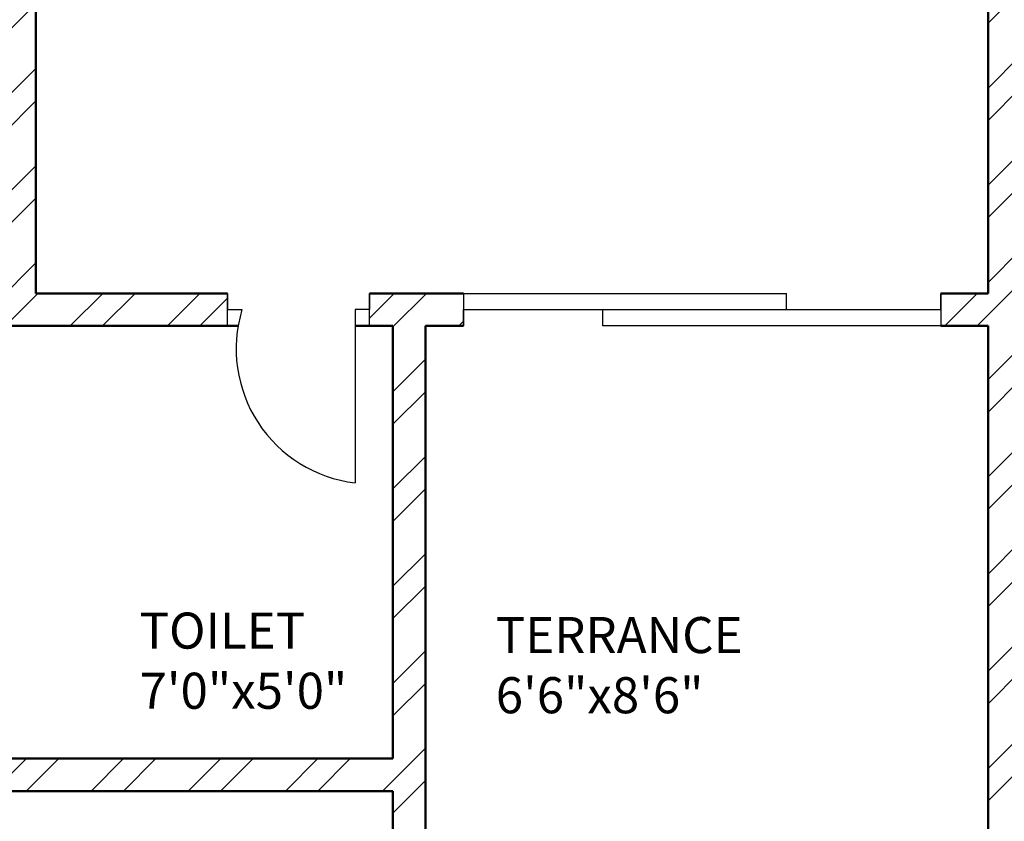
# Model space of a CAD drawing. Units: inches. Extents: x 963 to 2075, y 289 to 2657.
# Tile 5 of 98: x 1374 to 1511, y 1474 to 1585. Entities that reach past the tile are written whole.
import ezdxf

# ---------------------------------------------------------------- set-up
doc = ezdxf.new("R2010")
doc.units = ezdxf.units.IN
for name, color, linetype, lineweight in [('A-AREA-IDEN', 7, 'Continuous', 18), ('A-DOOR', 4, 'Continuous', 25), ('A-GLAZ', 3, 'Continuous', 25), ('A-WALL', 7, 'Continuous', 50), ('A-WALL-PATT', 8, 'Continuous', 13)]:
    doc.layers.add(name, color=color, linetype=linetype, lineweight=lineweight)
doc.styles.get("Standard").update_dxf_attribs({"font": 'arial.ttf'})

msp = doc.modelspace()

# ---------------------------------------------------------------- hatches: boundary and pattern name
at = {"layer": 'A-WALL-PATT'}
h = msp.add_hatch(dxfattribs=at)
h.set_pattern_fill('ANSI32', color=256)
h.paths.add_polyline_path([(1296.92, 2558.32), (1203.92, 2558.32), (1203.92, 2493.82), (1191.53, 2493.82), (1191.53, 2489.32), (1211.06, 2489.32), (1211.06, 2492.02), (1211.06, 2493.82), (1208.42, 2493.82), (1208.42, 2553.82), (1292.42, 2553.82), (1292.42, 2538.86), (1296.92, 2538.86)])
h.paths.add_polyline_path([(1442.42, 2558.32), (1349.42, 2558.32), (1349.42, 2538.94), (1353.92, 2538.94), (1353.92, 2553.82), (1437.92, 2553.82), (1437.92, 2493.82), (1434.54, 2493.82), (1434.54, 2489.32), (1448.31, 2489.32), (1448.31, 2491.57), (1448.31, 2493.82), (1442.42, 2493.82)])
h.paths.add_polyline_path([(1415.55, 2491.57), (1415.55, 2493.82), (1340.94, 2493.82), (1340.94, 2489.32), (1371.92, 2489.32), (1371.92, 2378.32), (1367.6, 2378.32), (1367.6, 2373.82), (1371.92, 2373.82), (1371.92, 2355.19), (1376.42, 2355.19), (1376.42, 2489.32), (1415.55, 2489.32)])
h.paths.add_polyline_path([(1304.94, 2491.57), (1304.94, 2493.82), (1296.92, 2493.82), (1296.92, 2514.86), (1292.42, 2514.86), (1292.42, 2493.82), (1232.81, 2493.82), (1232.81, 2489.32), (1256.42, 2489.32), (1256.42, 2327.32), (1253.71, 2327.32), (1253.71, 2322.82), (1328.42, 2322.82), (1328.42, 2331.15), (1323.92, 2331.15), (1323.92, 2327.32), (1260.92, 2327.32), (1260.92, 2373.82), (1323.92, 2373.82), (1323.92, 2357.81), (1328.42, 2357.81), (1328.42, 2373.82), (1346.01, 2373.82), (1346.01, 2376.07), (1346.01, 2378.32), (1260.92, 2378.32), (1260.92, 2489.32), (1304.94, 2489.32)])
h.paths.add_polyline_path([(1226.65, 2327.32), (1124.42, 2327.32), (1124.42, 2347.45), (1119.92, 2347.45), (1119.92, 2322.82), (1163.42, 2322.82), (1163.42, 2305.43), (1165.67, 2305.43), (1167.92, 2305.43), (1167.92, 2322.82), (1226.65, 2322.82), (1226.65, 2325.07)])
h.paths.add_polyline_path([(1095.92, 2489.32), (1124.42, 2489.32), (1131.53, 2489.32), (1131.53, 2491.57), (1131.53, 2493.82), (1119.92, 2493.82), (1091.42, 2493.82), (1091.42, 2417.32), (1095.92, 2417.32), (1119.92, 2417.32), (1119.92, 2407.45), (1124.42, 2407.45), (1124.42, 2421.82), (1095.92, 2421.82)])
h.paths.add_polyline_path([(1512.92, 2558.32), (1508.42, 2558.32), (1508.42, 2493.82), (1503.4, 2493.82), (1503.4, 2489.32), (1508.42, 2489.32), (1508.42, 2327.32), (1376.42, 2327.32), (1376.42, 2330.27), (1371.92, 2330.27), (1371.92, 2298.74), (1376.42, 2298.74), (1376.42, 2322.82), (1508.42, 2322.82), (1508.42, 2165.32), (1504.26, 2165.32), (1504.26, 2160.82), (1508.42, 2160.82), (1508.42, 2108.32), (1512.92, 2108.32), (1512.92, 2160.82), (1516.18, 2160.82), (1516.18, 2163.07), (1516.18, 2165.32), (1512.92, 2165.32), (1512.92, 2322.82), (1644.92, 2322.82), (1644.92, 2298.74), (1649.42, 2298.74), (1649.42, 2322.82), (1649.42, 2330.94), (1647.17, 2330.94), (1644.92, 2330.94), (1644.92, 2327.32), (1512.92, 2327.32), (1512.92, 2489.32), (1516.76, 2489.32), (1516.76, 2491.57), (1516.76, 2493.82), (1512.92, 2493.82)])
h.paths.add_polyline_path([(1671.92, 2558.32), (1578.92, 2558.32), (1578.92, 2493.82), (1573.53, 2493.82), (1573.53, 2489.32), (1586.54, 2489.32), (1586.54, 2491.57), (1586.54, 2493.82), (1583.42, 2493.82), (1583.42, 2553.82), (1667.42, 2553.82), (1667.42, 2541.11), (1671.92, 2541.11)])
h.paths.add_polyline_path([(1681.26, 2493.82), (1671.92, 2493.82), (1671.92, 2517.11), (1667.42, 2517.11), (1667.42, 2493.82), (1610.22, 2493.82), (1610.22, 2489.32), (1644.92, 2489.32), (1644.92, 2357.87), (1649.42, 2357.87), (1649.42, 2373.82), (1652.2, 2373.82), (1652.2, 2375.83), (1652.2, 2378.32), (1649.42, 2378.32), (1649.42, 2489.32), (1681.26, 2489.32), (1681.26, 2491.57)])
h.paths.add_polyline_path([(1821.92, 2558.32), (1728.92, 2558.32), (1728.92, 2541), (1733.42, 2541), (1733.42, 2553.82), (1817.42, 2553.82), (1817.42, 2493.82), (1813.51, 2493.82), (1813.51, 2489.32), (1830.08, 2489.32), (1830.08, 2491.57), (1830.08, 2493.82), (1821.92, 2493.82)])
h.paths.add_polyline_path([(1794.24, 2493.82), (1717.26, 2493.82), (1717.26, 2489.32), (1760.42, 2489.32), (1760.42, 2378.32), (1674.4, 2378.32), (1674.4, 2373.82), (1692.92, 2373.82), (1692.92, 2356.95), (1697.42, 2356.95), (1697.42, 2373.82), (1760.42, 2373.82), (1760.42, 2327.32), (1697.42, 2327.32), (1697.42, 2333.34), (1692.92, 2333.34), (1692.92, 2322.82), (1768.04, 2322.82), (1768.04, 2325.07), (1768.04, 2327.32), (1764.92, 2327.32), (1764.92, 2489.32), (1794.24, 2489.32)])
h.paths.add_polyline_path([(1733.42, 2517), (1728.92, 2517), (1728.92, 2493.82), (1733.42, 2493.82)], flags=17)
h.paths.add_polyline_path([(1929.92, 2493.82), (1890.08, 2493.82), (1890.08, 2489.32), (1896.92, 2489.32), (1925.42, 2489.32), (1925.42, 2421.82), (1896.92, 2421.82), (1896.92, 2408.32), (1901.42, 2408.32), (1901.42, 2417.32), (1925.42, 2417.32), (1929.92, 2417.32)])
h.paths.add_polyline_path([(1901.42, 2348.32), (1896.92, 2348.32), (1896.92, 2327.32), (1800.42, 2327.32), (1800.42, 2322.82), (1853.42, 2322.82), (1853.42, 2309.45), (1857.92, 2309.45), (1857.92, 2322.82), (1901.42, 2322.82)])
h.paths.add_polyline_path([(1857.92, 2249.45), (1853.42, 2249.45), (1853.42, 2214.82), (1686.31, 2214.82), (1686.31, 2210.32), (1853.42, 2210.32), (1853.42, 2202.13), (1857.92, 2202.13), (1857.92, 2210.32)])
h.paths.add_polyline_path([(1857.92, 2142.13), (1853.42, 2142.13), (1853.42, 2115.42), (1841.42, 2115.42), (1841.42, 2088.53), (1841.42, 2046.95), (1845.92, 2046.95), (1845.92, 2110.92), (1905.92, 2110.92), (1905.92, 2092.52), (1910.42, 2092.52), (1910.42, 2115.42), (1857.92, 2115.42)])
h.paths.add_polyline_path([(1532.44, 1482.34), (1573.46, 1482.34), (1573.46, 1501), (1532.44, 1501)], flags=9)
h.paths.add_polyline_path([(1438.66, 1486.3), (1479.68, 1486.3), (1479.68, 1504.96), (1438.66, 1504.96)], flags=9)
h.paths.add_polyline_path([(1411.22, 1365.31), (1659.14, 1365.31), (1659.14, 1402.4), (1411.22, 1402.4)], flags=9)
h.paths.add_polyline_path([(1185.67, 2296.3), (1248.16, 2296.3), (1248.16, 2314.95), (1185.67, 2314.95)], flags=9)
h.paths.add_polyline_path([(1177.31, 2187.35), (1216.15, 2187.35), (1216.15, 2206.01), (1177.31, 2206.01)], flags=9)
h.paths.add_polyline_path([(1295.1, 1602.08), (1328.26, 1602.08), (1328.26, 1620.74), (1295.1, 1620.74)], flags=9)
h.paths.add_polyline_path([(1525.13, 2005.99), (1558.39, 2005.99), (1558.39, 2024.65), (1525.13, 2024.65)], flags=9)
h.paths.add_polyline_path([(1459.61, 1977.13), (1472.19, 1977.13), (1472.19, 1987.43), (1459.61, 1987.43)], flags=9)
h.paths.add_polyline_path([(1467.81, 2053.68), (1480.02, 2053.68), (1480.02, 2063.98), (1467.81, 2063.98)], flags=9)
h.paths.add_polyline_path([(1555.18, 2119.02), (1584.56, 2119.02), (1584.56, 2137.68), (1555.18, 2137.68)], flags=25)
h.paths.add_polyline_path([(1405.39, 2115.29), (1444.48, 2115.29), (1444.48, 2133.95), (1405.39, 2133.95)], flags=25)
h.paths.add_polyline_path([(1698.48, 2004.26), (1727.69, 2004.26), (1727.69, 2022.92), (1698.48, 2022.92)], flags=9)
h.paths.add_polyline_path([(1612.16, 1972.86), (1629.02, 1972.86), (1629.02, 1983.16), (1612.16, 1983.16)], flags=9)
h.paths.add_polyline_path([(1608.29, 2060.04), (1625.15, 2060.04), (1625.15, 2070.34), (1608.29, 2070.34)], flags=9)
h.paths.add_polyline_path([(1527.95, 1684.4), (1566.79, 1684.4), (1566.79, 1703.06), (1527.95, 1703.06)], flags=9)
h.paths.add_polyline_path([(1422.79, 1683.59), (1461.63, 1683.59), (1461.63, 1702.25), (1422.79, 1702.25)], flags=9)
h.paths.add_polyline_path([(1531.26, 1732.46), (1574.01, 1732.46), (1574.01, 1751.12), (1531.26, 1751.12)], flags=9)
h.paths.add_polyline_path([(1402.87, 1732.85), (1439.8, 1732.85), (1439.8, 1751.5), (1402.87, 1751.5)], flags=9)
h.paths.add_polyline_path([(1243.12, 1923.13), (1281.96, 1923.13), (1281.96, 1941.79), (1243.12, 1941.79)], flags=9)
h.paths.add_polyline_path([(1181.75, 1792.27), (1244.24, 1792.27), (1244.24, 1810.93), (1181.75, 1810.93)], flags=9)
h.paths.add_polyline_path([(1265.82, 1670.3), (1316.07, 1670.3), (1316.07, 1688.96), (1265.82, 1688.96)], flags=9)
h.paths.add_polyline_path([(1140.26, 1676.05), (1179.1, 1676.05), (1179.1, 1694.71), (1140.26, 1694.71)], flags=9)
h.paths.add_polyline_path([(1107.49, 1490.89), (1143.37, 1490.89), (1143.37, 1509.55), (1107.49, 1509.55)], flags=9)
h.paths.add_polyline_path([(1217.58, 1483.9), (1246.74, 1483.9), (1246.74, 1502.56), (1217.58, 1502.56)], flags=9)
h.paths.add_polyline_path([(1389.21, 1486.92), (1418.37, 1486.92), (1418.37, 1505.58), (1389.21, 1505.58)], flags=9)
h.paths.add_polyline_path([(1672.21, 1602.08), (1705.37, 1602.08), (1705.37, 1620.74), (1672.21, 1620.74)], flags=9)
h.paths.add_polyline_path([(1752.08, 1522.64), (1781.24, 1522.64), (1781.24, 1541.3), (1752.08, 1541.3)], flags=9)
h.paths.add_polyline_path([(1848.27, 1491.26), (1884.16, 1491.26), (1884.16, 1509.92), (1848.27, 1509.92)], flags=9)
h.paths.add_polyline_path([(1822.47, 1685.62), (1861.31, 1685.62), (1861.31, 1704.28), (1822.47, 1704.28)], flags=9)
h.paths.add_polyline_path([(1713.19, 1672.23), (1763.44, 1672.23), (1763.44, 1690.89), (1713.19, 1690.89)], flags=9)
h.paths.add_polyline_path([(1736.62, 1790.58), (1799.11, 1790.58), (1799.11, 1809.24), (1736.62, 1809.24)], flags=9)
h.paths.add_polyline_path([(1691.49, 1916.36), (1730.33, 1916.36), (1730.33, 1935.01), (1691.49, 1935.01)], flags=9)
h.paths.add_polyline_path([(1764.87, 1973.92), (1794.31, 1973.92), (1794.31, 1992.58), (1764.87, 1992.58)], flags=9)
h.paths.add_polyline_path([(1767.85, 2034.02), (1797.29, 2034.02), (1797.29, 2052.67), (1767.85, 2052.67)], flags=9)
h.paths.add_polyline_path([(1851.59, 2060.33), (1880.75, 2060.33), (1880.75, 2078.99), (1851.59, 2078.99)], flags=25)
h.paths.add_polyline_path([(1688.49, 2086.87), (1727.33, 2086.87), (1727.33, 2105.53), (1688.49, 2105.53)], flags=9)
h.paths.add_polyline_path([(1537.74, 2293.58), (1580.49, 2293.58), (1580.49, 2312.24), (1537.74, 2312.24)], flags=25)
h.paths.add_polyline_path([(1425.59, 2296.11), (1468.34, 2296.11), (1468.34, 2314.77), (1425.59, 2314.77)], flags=25)
h.paths.add_polyline_path([(1278.52, 2004.18), (1307.72, 2004.18), (1307.72, 2022.84), (1278.52, 2022.84)], flags=9)
h.paths.add_polyline_path([(1193.28, 1973.63), (1222.72, 1973.63), (1222.72, 1992.29), (1193.28, 1992.29)], flags=9)
h.paths.add_polyline_path([(1192.41, 2040.58), (1221.84, 2040.58), (1221.84, 2059.23), (1192.41, 2059.23)], flags=9)
h.paths.add_polyline_path([(1130.6, 1951.39), (1159.76, 1951.39), (1159.76, 1970.05), (1130.6, 1970.05)], flags=9)
h.paths.add_polyline_path([(1132.83, 2052.49), (1161.98, 2052.49), (1161.98, 2071.15), (1132.83, 2071.15)], flags=9)
h.paths.add_polyline_path([(1265.13, 2334.62), (1315.38, 2334.62), (1315.38, 2353.28), (1265.13, 2353.28)], flags=25)
h.paths.add_polyline_path([(1136.74, 2330.79), (1175.58, 2330.79), (1175.58, 2349.44), (1136.74, 2349.44)], flags=9)
h.paths.add_polyline_path([(1287.42, 2417.2), (1320.58, 2417.2), (1320.58, 2435.86), (1287.42, 2435.86)], flags=25)
h.paths.add_polyline_path([(1430.99, 2329.16), (1469.83, 2329.16), (1469.83, 2347.82), (1430.99, 2347.82)], flags=25)
h.paths.add_polyline_path([(1525.42, 2329.21), (1564.26, 2329.21), (1564.26, 2347.87), (1525.42, 2347.87)], flags=25)
h.paths.add_polyline_path([(1684.52, 2382.8), (1717.68, 2382.8), (1717.68, 2401.46), (1684.52, 2401.46)], flags=25)
h.paths.add_polyline_path([(1704.81, 2340.29), (1755.05, 2340.29), (1755.05, 2358.95), (1704.81, 2358.95)], flags=25)
h.paths.add_polyline_path([(1694.11, 2287.76), (1756.6, 2287.76), (1756.6, 2306.41), (1694.11, 2306.41)], flags=9)
h.paths.add_polyline_path([(1815.78, 2329.86), (1854.62, 2329.86), (1854.62, 2348.52), (1815.78, 2348.52)], flags=9)
h.paths.add_polyline_path([(1842.87, 2514.26), (1878.76, 2514.26), (1878.76, 2532.91), (1842.87, 2532.91)], flags=9)
h.paths.add_polyline_path([(1769.51, 2531.45), (1798.67, 2531.45), (1798.67, 2550.1), (1769.51, 2550.1)], flags=25)
h.paths.add_polyline_path([(1594.77, 2518.47), (1623.93, 2518.47), (1623.93, 2537.13), (1594.77, 2537.13)], flags=25)
h.paths.add_polyline_path([(1520.72, 2516.18), (1556.61, 2516.18), (1556.61, 2534.84), (1520.72, 2534.84)], flags=25)
h.paths.add_polyline_path([(1464.46, 2516.69), (1500.34, 2516.69), (1500.34, 2535.35), (1464.46, 2535.35)], flags=25)
h.paths.add_polyline_path([(1365.7, 2528.97), (1394.85, 2528.97), (1394.85, 2547.63), (1365.7, 2547.63)], flags=25)
h.paths.add_polyline_path([(1222.84, 2516.23), (1252, 2516.23), (1252, 2534.89), (1222.84, 2534.89)], flags=25)
h.paths.add_polyline_path([(1104.55, 2509.6), (1140.43, 2509.6), (1140.43, 2528.26), (1104.55, 2528.26)], flags=9)
h = msp.add_hatch(dxfattribs=at)
h.set_pattern_fill('ANSI32', color=256)
h.paths.add_polyline_path([(1335.97, 2212.57), (1335.97, 2214.82), (1167.92, 2214.82), (1167.92, 2245.43), (1163.42, 2245.43), (1163.42, 2210.32), (1163.42, 2194.81), (1167.92, 2194.81), (1167.92, 2210.32), (1335.97, 2210.32)])
h.paths.add_polyline_path([(1532.44, 1482.34), (1573.46, 1482.34), (1573.46, 1501), (1532.44, 1501)], flags=9)
h.paths.add_polyline_path([(1438.66, 1486.3), (1479.68, 1486.3), (1479.68, 1504.96), (1438.66, 1504.96)], flags=9)
h.paths.add_polyline_path([(1411.22, 1365.31), (1659.14, 1365.31), (1659.14, 1402.4), (1411.22, 1402.4)], flags=9)
h.paths.add_polyline_path([(1185.67, 2296.3), (1248.16, 2296.3), (1248.16, 2314.95), (1185.67, 2314.95)], flags=9)
h.paths.add_polyline_path([(1177.31, 2187.35), (1216.15, 2187.35), (1216.15, 2206.01), (1177.31, 2206.01)], flags=9)
h.paths.add_polyline_path([(1295.1, 1602.08), (1328.26, 1602.08), (1328.26, 1620.74), (1295.1, 1620.74)], flags=9)
h.paths.add_polyline_path([(1525.13, 2005.99), (1558.39, 2005.99), (1558.39, 2024.65), (1525.13, 2024.65)], flags=9)
h.paths.add_polyline_path([(1459.61, 1977.13), (1472.19, 1977.13), (1472.19, 1987.43), (1459.61, 1987.43)], flags=9)
h.paths.add_polyline_path([(1467.81, 2053.68), (1480.02, 2053.68), (1480.02, 2063.98), (1467.81, 2063.98)], flags=9)
h.paths.add_polyline_path([(1555.18, 2119.02), (1584.56, 2119.02), (1584.56, 2137.68), (1555.18, 2137.68)], flags=9)
h.paths.add_polyline_path([(1405.39, 2115.29), (1444.48, 2115.29), (1444.48, 2133.95), (1405.39, 2133.95)], flags=9)
h.paths.add_polyline_path([(1698.48, 2004.26), (1727.69, 2004.26), (1727.69, 2022.92), (1698.48, 2022.92)], flags=9)
h.paths.add_polyline_path([(1612.16, 1972.86), (1629.02, 1972.86), (1629.02, 1983.16), (1612.16, 1983.16)], flags=9)
h.paths.add_polyline_path([(1608.29, 2060.04), (1625.15, 2060.04), (1625.15, 2070.34), (1608.29, 2070.34)], flags=9)
h.paths.add_polyline_path([(1527.95, 1684.4), (1566.79, 1684.4), (1566.79, 1703.06), (1527.95, 1703.06)], flags=9)
h.paths.add_polyline_path([(1422.79, 1683.59), (1461.63, 1683.59), (1461.63, 1702.25), (1422.79, 1702.25)], flags=9)
h.paths.add_polyline_path([(1531.26, 1732.46), (1574.01, 1732.46), (1574.01, 1751.12), (1531.26, 1751.12)], flags=9)
h.paths.add_polyline_path([(1402.87, 1732.85), (1439.8, 1732.85), (1439.8, 1751.5), (1402.87, 1751.5)], flags=9)
h.paths.add_polyline_path([(1243.12, 1923.13), (1281.96, 1923.13), (1281.96, 1941.79), (1243.12, 1941.79)], flags=9)
h.paths.add_polyline_path([(1181.75, 1792.27), (1244.24, 1792.27), (1244.24, 1810.93), (1181.75, 1810.93)], flags=9)
h.paths.add_polyline_path([(1265.82, 1670.3), (1316.07, 1670.3), (1316.07, 1688.96), (1265.82, 1688.96)], flags=9)
h.paths.add_polyline_path([(1140.26, 1676.05), (1179.1, 1676.05), (1179.1, 1694.71), (1140.26, 1694.71)], flags=9)
h.paths.add_polyline_path([(1107.49, 1490.89), (1143.37, 1490.89), (1143.37, 1509.55), (1107.49, 1509.55)], flags=9)
h.paths.add_polyline_path([(1217.58, 1483.9), (1246.74, 1483.9), (1246.74, 1502.56), (1217.58, 1502.56)], flags=9)
h.paths.add_polyline_path([(1389.21, 1486.92), (1418.37, 1486.92), (1418.37, 1505.58), (1389.21, 1505.58)], flags=9)
h.paths.add_polyline_path([(1672.21, 1602.08), (1705.37, 1602.08), (1705.37, 1620.74), (1672.21, 1620.74)], flags=9)
h.paths.add_polyline_path([(1752.08, 1522.64), (1781.24, 1522.64), (1781.24, 1541.3), (1752.08, 1541.3)], flags=9)
h.paths.add_polyline_path([(1848.27, 1491.26), (1884.16, 1491.26), (1884.16, 1509.92), (1848.27, 1509.92)], flags=9)
h.paths.add_polyline_path([(1822.47, 1685.62), (1861.31, 1685.62), (1861.31, 1704.28), (1822.47, 1704.28)], flags=9)
h.paths.add_polyline_path([(1713.19, 1672.23), (1763.44, 1672.23), (1763.44, 1690.89), (1713.19, 1690.89)], flags=9)
h.paths.add_polyline_path([(1736.62, 1790.58), (1799.11, 1790.58), (1799.11, 1809.24), (1736.62, 1809.24)], flags=9)
h.paths.add_polyline_path([(1691.49, 1916.36), (1730.33, 1916.36), (1730.33, 1935.01), (1691.49, 1935.01)], flags=9)
h.paths.add_polyline_path([(1764.87, 1973.92), (1794.31, 1973.92), (1794.31, 1992.58), (1764.87, 1992.58)], flags=9)
h.paths.add_polyline_path([(1767.85, 2034.02), (1797.29, 2034.02), (1797.29, 2052.67), (1767.85, 2052.67)], flags=9)
h.paths.add_polyline_path([(1851.59, 2060.33), (1880.75, 2060.33), (1880.75, 2078.99), (1851.59, 2078.99)], flags=9)
h.paths.add_polyline_path([(1688.49, 2086.87), (1727.33, 2086.87), (1727.33, 2105.53), (1688.49, 2105.53)], flags=9)
h.paths.add_polyline_path([(1537.74, 2293.58), (1580.49, 2293.58), (1580.49, 2312.24), (1537.74, 2312.24)], flags=9)
h.paths.add_polyline_path([(1425.59, 2296.11), (1468.34, 2296.11), (1468.34, 2314.77), (1425.59, 2314.77)], flags=9)
h.paths.add_polyline_path([(1278.52, 2004.18), (1307.72, 2004.18), (1307.72, 2022.84), (1278.52, 2022.84)], flags=9)
h.paths.add_polyline_path([(1193.28, 1973.63), (1222.72, 1973.63), (1222.72, 1992.29), (1193.28, 1992.29)], flags=9)
h.paths.add_polyline_path([(1192.41, 2040.58), (1221.84, 2040.58), (1221.84, 2059.23), (1192.41, 2059.23)], flags=9)
h.paths.add_polyline_path([(1130.6, 1951.39), (1159.76, 1951.39), (1159.76, 1970.05), (1130.6, 1970.05)], flags=9)
h.paths.add_polyline_path([(1132.83, 2052.49), (1161.98, 2052.49), (1161.98, 2071.15), (1132.83, 2071.15)], flags=9)
h.paths.add_polyline_path([(1265.13, 2334.62), (1315.38, 2334.62), (1315.38, 2353.28), (1265.13, 2353.28)], flags=9)
h.paths.add_polyline_path([(1136.74, 2330.79), (1175.58, 2330.79), (1175.58, 2349.44), (1136.74, 2349.44)], flags=9)
h.paths.add_polyline_path([(1287.42, 2417.2), (1320.58, 2417.2), (1320.58, 2435.86), (1287.42, 2435.86)], flags=9)
h.paths.add_polyline_path([(1430.99, 2329.16), (1469.83, 2329.16), (1469.83, 2347.82), (1430.99, 2347.82)], flags=9)
h.paths.add_polyline_path([(1525.42, 2329.21), (1564.26, 2329.21), (1564.26, 2347.87), (1525.42, 2347.87)], flags=9)
h.paths.add_polyline_path([(1684.52, 2382.8), (1717.68, 2382.8), (1717.68, 2401.46), (1684.52, 2401.46)], flags=9)
h.paths.add_polyline_path([(1704.81, 2340.29), (1755.05, 2340.29), (1755.05, 2358.95), (1704.81, 2358.95)], flags=9)
h.paths.add_polyline_path([(1694.11, 2287.76), (1756.6, 2287.76), (1756.6, 2306.41), (1694.11, 2306.41)], flags=9)
h.paths.add_polyline_path([(1815.78, 2329.86), (1854.62, 2329.86), (1854.62, 2348.52), (1815.78, 2348.52)], flags=9)
h.paths.add_polyline_path([(1842.87, 2514.26), (1878.76, 2514.26), (1878.76, 2532.91), (1842.87, 2532.91)], flags=9)
h.paths.add_polyline_path([(1769.51, 2531.45), (1798.67, 2531.45), (1798.67, 2550.1), (1769.51, 2550.1)], flags=9)
h.paths.add_polyline_path([(1594.77, 2518.47), (1623.93, 2518.47), (1623.93, 2537.13), (1594.77, 2537.13)], flags=9)
h.paths.add_polyline_path([(1520.72, 2516.18), (1556.61, 2516.18), (1556.61, 2534.84), (1520.72, 2534.84)], flags=9)
h.paths.add_polyline_path([(1464.46, 2516.69), (1500.34, 2516.69), (1500.34, 2535.35), (1464.46, 2535.35)], flags=9)
h.paths.add_polyline_path([(1365.7, 2528.97), (1394.85, 2528.97), (1394.85, 2547.63), (1365.7, 2547.63)], flags=9)
h.paths.add_polyline_path([(1222.84, 2516.23), (1252, 2516.23), (1252, 2534.89), (1222.84, 2534.89)], flags=9)
h.paths.add_polyline_path([(1104.55, 2509.6), (1140.43, 2509.6), (1140.43, 2528.26), (1104.55, 2528.26)], flags=9)
h = msp.add_hatch(dxfattribs=at)
h.set_pattern_fill('ANSI32', color=256)
h.paths.add_polyline_path([(1473.61, 2163.07), (1473.61, 2165.32), (1376.42, 2165.32), (1376.42, 2227.98), (1371.92, 2227.98), (1371.92, 2214.82), (1368.41, 2214.82), (1368.41, 2210.32), (1371.92, 2210.32), (1371.92, 2160.82), (1395.92, 2160.82), (1395.92, 2090.32), (1217.34, 2090.32), (1217.34, 2085.82), (1395.92, 2085.82), (1458.92, 2085.82), (1458.92, 2108.32), (1454.42, 2108.32), (1454.42, 2090.32), (1400.42, 2090.32), (1400.42, 2160.82), (1473.61, 2160.82)])
h.paths.add_polyline_path([(1649.42, 2210.32), (1653.23, 2210.32), (1653.23, 2214.82), (1649.42, 2214.82), (1649.42, 2227.98), (1644.92, 2227.98), (1644.92, 2165.32), (1550.1, 2165.32), (1550.1, 2160.82), (1620.92, 2160.82), (1620.92, 2112.82), (1555.45, 2112.82), (1555.45, 2108.32), (1584.33, 2108.32), (1584.33, 2084.92), (1588.83, 2084.92), (1588.83, 2108.32), (1625.42, 2108.32), (1667.95, 2108.32), (1667.95, 2022.67), (1588.83, 2022.67), (1588.83, 2047.41), (1584.33, 2047.41), (1584.33, 1996), (1588.83, 1996), (1588.83, 2018.32), (1667.95, 2018.17), (1667.95, 1928.32), (1625.42, 1928.32), (1625.42, 1923.82), (1672.45, 1923.82), (1672.45, 1928.32), (1672.45, 1946.66), (1785.45, 1946.66), (1785.45, 1951.16), (1743.03, 1951.16), (1743.03, 2017.92), (1841.42, 2017.92), (1841.42, 2014.77), (1845.92, 2014.77), (1845.92, 2017.92), (1905.92, 2017.92), (1905.92, 1987.51), (1910.42, 1987.51), (1910.42, 2022.42), (1910.42, 2068.52), (1905.92, 2068.52), (1905.92, 2022.42), (1845.92, 2022.42), (1845.92, 2025.85), (1843.67, 2025.85), (1841.42, 2025.85), (1841.42, 2022.42), (1743.03, 2022.42), (1743.03, 2084.03), (1768.45, 2084.03), (1785.45, 2084.03), (1785.45, 2088.53), (1672.45, 2088.53), (1672.45, 2112.82), (1667.95, 2112.82), (1625.42, 2112.82), (1625.42, 2160.82), (1649.42, 2160.82)])
h.paths.add_polyline_path([(1672.45, 2084.03), (1738.53, 2084.03), (1738.53, 1951.16), (1672.45, 1951.16)], flags=16)
h.paths.add_polyline_path([(1672.45, 2084.03), (1738.53, 2084.03), (1705.49, 2017.6)], flags=0)
h.paths.add_polyline_path([(1262.77, 2085.82), (1258.27, 2085.82), (1258.27, 2023.28), (1184.42, 2023.28), (1184.42, 2018.78), (1258.27, 2018.78), (1258.27, 1950.82), (1262.77, 1950.82)])
h.paths.add_polyline_path([(1312.27, 2085.82), (1307.77, 2085.82), (1307.77, 1950.82), (1312.27, 1950.82)])
h.paths.add_polyline_path([(1458.92, 1950.82), (1395.92, 1950.82), (1216.57, 1950.82), (1216.57, 1946.32), (1346.42, 1946.32), (1395.92, 1946.32), (1395.92, 1875.82), (1371.92, 1875.82), (1371.92, 1826.32), (1368.93, 1826.32), (1368.93, 1821.82), (1371.92, 1821.82), (1371.92, 1813.62), (1376.42, 1813.62), (1376.42, 1871.32), (1474.5, 1871.32), (1474.5, 1873.57), (1474.5, 1875.82), (1400.42, 1875.82), (1400.42, 1946.32), (1454.42, 1946.32), (1454.42, 1928.32), (1458.92, 1928.32)])
h.paths.add_polyline_path([(1184.42, 2120.78), (1167.92, 2120.78), (1167.92, 2134.81), (1165.67, 2134.81), (1163.42, 2134.81), (1163.42, 2120.78), (1119.92, 2120.78), (1119.92, 2098.1), (1124.42, 2098.1), (1124.42, 2116.28), (1167.92, 2116.28), (1179.92, 2116.28), (1179.92, 2045.92), (1184.42, 2045.92), (1184.42, 2090.32), (1184.42, 2116.28)])
h.paths.add_polyline_path([(1124.42, 2018.78), (1179.92, 2018.78), (1179.92, 2016.29), (1184.42, 2016.29), (1184.42, 2023.28), (1184.42, 2026.59), (1182.17, 2026.59), (1179.92, 2026.59), (1179.92, 2023.28), (1124.42, 2023.28), (1124.42, 2074.1), (1119.92, 2074.1), (1119.92, 2018.78), (1119.92, 1979.63), (1124.42, 1979.63)])
h.paths.add_polyline_path([(1184.42, 1925.78), (1184.42, 1946.32), (1184.42, 1996.07), (1182.17, 1996.07), (1179.92, 1996.07), (1179.92, 1925.78), (1124.42, 1925.78), (1124.42, 1955.63), (1119.92, 1955.5), (1119.92, 1921.28), (1158.92, 1921.28), (1158.92, 1909.98), (1163.42, 1909.98), (1163.42, 1921.28), (1184.42, 1921.28)])
h.paths.add_polyline_path([(1341.45, 1826.32), (1163.42, 1826.32), (1163.42, 1849.98), (1158.92, 1849.98), (1158.92, 1821.82), (1158.92, 1804.03), (1163.42, 1804.03), (1163.42, 1821.82), (1341.45, 1821.82)])
h.paths.add_polyline_path([(1222.98, 1713.82), (1163.42, 1713.82), (1163.42, 1744.03), (1161.17, 1744.03), (1158.92, 1744.03), (1158.92, 1713.82), (1119.92, 1713.82), (1119.92, 1694.65), (1124.42, 1694.65), (1124.42, 1709.32), (1158.92, 1709.32), (1222.98, 1709.32)])
h.paths.add_polyline_path([(1328.42, 1713.82), (1252.04, 1713.82), (1252.04, 1711.57), (1252.04, 1709.32), (1256.42, 1709.32), (1256.42, 1547.32), (1232.94, 1547.32), (1232.94, 1545.07), (1232.94, 1542.82), (1292.42, 1542.82), (1292.42, 1527.63), (1296.92, 1527.63), (1296.92, 1542.82), (1299.46, 1542.82), (1299.46, 1547.32), (1260.92, 1547.32), (1260.92, 1658.32), (1343.66, 1658.32), (1343.66, 1660.57), (1343.66, 1662.82), (1328.42, 1662.82), (1328.42, 1676.59), (1327.4, 1676.59), (1323.92, 1676.59), (1323.92, 1662.82), (1260.92, 1662.82), (1260.92, 1709.32), (1323.92, 1709.32), (1323.92, 1699.85), (1328.42, 1699.85)])
h.paths.add_polyline_path([(1649.42, 1875.82), (1625.42, 1875.82), (1625.42, 1928.32), (1620.92, 1928.32), (1588.83, 1928.32), (1588.83, 1950.59), (1584.33, 1950.59), (1584.33, 1928.32), (1555.45, 1928.32), (1555.45, 1923.82), (1620.92, 1923.82), (1620.92, 1875.82), (1548.95, 1875.82), (1548.95, 1873.57), (1548.95, 1871.32), (1644.92, 1871.32), (1644.92, 1813.62), (1649.42, 1813.62), (1649.42, 1821.82), (1652.04, 1821.82), (1652.04, 1824.07), (1652.04, 1826.32), (1649.42, 1826.32)])
h.paths.add_polyline_path([(1512.92, 1871.32), (1516.48, 1871.32), (1516.48, 1875.82), (1512.92, 1875.82), (1512.92, 1923.82), (1512.92, 1928.32), (1512.92, 1930.83), (1508.42, 1930.83), (1508.42, 1875.82), (1504.41, 1875.82), (1504.41, 1871.32), (1508.42, 1871.32), (1508.42, 1713.82), (1376.42, 1713.82), (1376.42, 1743.32), (1371.92, 1743.32), (1371.92, 1709.32), (1371.92, 1706.01), (1376.42, 1706.01), (1376.42, 1709.32), (1508.42, 1709.32), (1508.42, 1547.32), (1501.87, 1547.32), (1501.87, 1542.82), (1508.42, 1542.82), (1508.42, 1482.82), (1508.42, 1436.32), (1512.92, 1436.32), (1512.92, 1542.82), (1519.32, 1542.82), (1519.32, 1545.07), (1519.32, 1547.32), (1512.92, 1547.32), (1512.92, 1709.32), (1644.92, 1709.32), (1644.92, 1707.55), (1649.42, 1707.55), (1649.42, 1709.32), (1649.42, 1743.32), (1644.92, 1743.32), (1644.92, 1713.82), (1512.92, 1713.82)])
h.paths.add_polyline_path([(1129.88, 1545.07), (1129.88, 1547.32), (1124.42, 1547.32), (1095.92, 1547.32), (1095.92, 1614.82), (1124.42, 1614.82), (1124.42, 1619.32), (1095.92, 1619.32), (1091.42, 1619.32), (1091.42, 1542.82), (1095.92, 1542.82), (1119.92, 1542.82), (1129.88, 1542.82)])
h.paths.add_polyline_path([(1208.42, 1542.82), (1211.74, 1542.82), (1211.74, 1547.32), (1198.85, 1547.32), (1198.85, 1542.82), (1203.92, 1542.82), (1203.92, 1478.32), (1208.42, 1478.32), (1296.92, 1478.32), (1296.92, 1503.63), (1292.42, 1503.63), (1292.42, 1482.82), (1208.42, 1482.82)])
h.paths.add_polyline_path([(1430.42, 1542.82), (1435.7, 1542.82), (1435.7, 1545.07), (1435.7, 1547.32), (1422.66, 1547.32), (1422.66, 1545.07), (1422.66, 1542.82), (1425.92, 1542.82), (1425.92, 1482.86), (1341.92, 1482.86), (1341.92, 1502.73), (1337.42, 1502.73), (1337.42, 1478.36), (1425.92, 1478.36), (1425.92, 1440.82), (1425.92, 1436.32), (1430.42, 1436.32)])
h.paths.add_polyline_path([(1698.48, 2004.26), (1727.69, 2004.26), (1727.69, 2022.92), (1698.48, 2022.92)], flags=8)
h = msp.add_hatch(dxfattribs=at)
h.set_pattern_fill('ANSI32', color=256)
h.paths.add_polyline_path([(1910.42, 1929.42), (1910.42, 1963.51), (1905.92, 1963.51), (1905.92, 1929.42), (1845.92, 1929.42), (1845.92, 1993.37), (1843.67, 1993.37), (1841.42, 1993.37), (1841.42, 1951.16), (1841.42, 1924.92), (1853.42, 1924.92), (1853.42, 1913.07), (1857.92, 1913.07), (1857.92, 1924.92), (1910.42, 1924.92)])
h.paths.add_polyline_path([(1857.92, 1853.07), (1853.42, 1853.07), (1853.42, 1826.32), (1841.42, 1826.32), (1674.48, 1826.32), (1674.48, 1821.82), (1853.42, 1821.82), (1857.92, 1821.82)])
h.paths.add_polyline_path([(1857.92, 1821.82), (1853.42, 1821.82), (1853.42, 1807.79), (1857.92, 1807.79)])
h.paths.add_polyline_path([(1857.92, 1747.79), (1853.42, 1747.79), (1853.42, 1713.82), (1809.34, 1713.82), (1809.34, 1709.32), (1905.92, 1709.32), (1905.92, 1688.32), (1910.42, 1688.32), (1910.42, 1713.82), (1857.92, 1713.82)])
h.paths.add_polyline_path([(1830.92, 1542.82), (1837.43, 1542.82), (1837.43, 1545.07), (1837.43, 1547.32), (1823.42, 1547.32), (1823.42, 1545.07), (1823.42, 1542.82), (1826.42, 1542.82), (1826.42, 1482.82), (1742.42, 1482.82), (1742.42, 1505.39), (1737.92, 1505.39), (1737.92, 1478.32), (1830.92, 1478.32)])
h.paths.add_polyline_path([(1938.92, 1619.32), (1934.42, 1619.32), (1910.42, 1619.32), (1910.42, 1628.32), (1908.17, 1628.32), (1905.92, 1628.32), (1905.92, 1614.82), (1934.42, 1614.82), (1934.42, 1547.32), (1905.92, 1547.32), (1899.59, 1547.32), (1899.59, 1542.82), (1910.42, 1542.82), (1938.92, 1542.82)])
h.paths.add_polyline_path([(1803.68, 1547.32), (1773.92, 1547.32), (1773.92, 1709.32), (1777.76, 1709.32), (1777.76, 1713.82), (1701.92, 1713.82), (1701.92, 1697.8), (1706.42, 1697.8), (1706.42, 1709.32), (1769.42, 1709.32), (1769.42, 1662.82), (1706.42, 1662.82), (1706.42, 1674.38), (1701.92, 1674.38), (1701.92, 1662.82), (1675.67, 1662.82), (1675.67, 1658.32), (1769.42, 1658.32), (1769.42, 1547.32), (1729.17, 1547.32), (1729.17, 1542.82), (1737.92, 1542.82), (1737.92, 1529.39), (1742.42, 1529.39), (1742.42, 1542.82), (1803.68, 1542.82)])
h.paths.add_polyline_path([(1595.42, 1542.82), (1599.24, 1542.82), (1599.24, 1547.32), (1584.36, 1547.32), (1584.36, 1542.82), (1590.92, 1542.82), (1590.92, 1436.32), (1595.42, 1436.32), (1595.42, 1440.82)])
h.paths.add_polyline_path([(1693.17, 1547.32), (1649.42, 1547.32), (1649.42, 1658.32), (1652.1, 1658.32), (1652.1, 1660.57), (1652.1, 1662.82), (1649.42, 1662.82), (1649.42, 1680.94), (1647.17, 1680.94), (1644.92, 1680.94), (1644.92, 1547.32), (1622.42, 1547.32), (1622.42, 1545.07), (1622.42, 1542.82), (1649.42, 1542.82), (1679.42, 1542.82), (1679.42, 1529.85), (1681.67, 1529.85), (1683.92, 1529.85), (1683.92, 1542.82), (1693.17, 1542.82), (1693.17, 1545.07)])
h.paths.add_polyline_path([(1683.92, 1505.85), (1679.42, 1505.85), (1679.42, 1483.8), (1595.42, 1483.8), (1595.42, 1479.3), (1683.92, 1479.3)])
h.paths.add_polyline_path([(1402.99, 1547.32), (1376.42, 1547.32), (1376.42, 1675.89), (1374.17, 1675.89), (1371.92, 1675.89), (1371.92, 1662.82), (1368.88, 1662.82), (1368.88, 1658.32), (1371.92, 1658.32), (1371.92, 1547.32), (1335.46, 1547.32), (1335.46, 1542.82), (1337.42, 1542.82), (1337.42, 1526.73), (1341.92, 1526.73), (1341.92, 1542.82), (1371.92, 1542.82), (1402.99, 1542.82)])

# ---------------------------------------------------------------- linework, layer by layer
at = {"layer": 'A-DOOR'}
for p, q in [((1402.99, 1542.82), (1402.99, 1547.32)), ((1402.99, 1547.32), (1402.99, 1545.07)), ((1422.66, 1542.82), (1422.66, 1547.32)), ((1422.66, 1547.32), (1422.66, 1545.07)), ((1402.99, 1545.07), (1404.99, 1545.07)), ((1422.66, 1545.07), (1420.66, 1545.07)), ((1420.66, 1545.07), (1420.66, 1521.07))]:
    msp.add_line(p, q, dxfattribs=at)
msp.add_arc((1422.87, 1539.62), 18.69, 163.0621, 263.2025, dxfattribs=at)
at = {"layer": 'A-GLAZ'}
for p, q in [((1435.7, 1547.32), (1435.7, 1542.82)), ((1435.7, 1547.32), (1480.49, 1547.32)), ((1480.49, 1545.07), (1480.49, 1547.32)), ((1501.87, 1545.07), (1501.87, 1547.32)), ((1501.87, 1547.32), (1501.87, 1542.82)), ((1435.7, 1542.82), (1435.7, 1545.07)), ((1435.7, 1545.07), (1501.87, 1545.07)), ((1455.01, 1542.82), (1455.01, 1545.07)), ((1501.87, 1542.82), (1455.01, 1542.82))]:
    msp.add_line(p, q, dxfattribs=at)
at = {"layer": 'A-WALL'}
for p, q in [((1508.42, 1709.32), (1508.42, 1547.32)), ((1376.42, 1677.26), (1376.42, 1547.32)), ((1402.99, 1547.32), (1376.42, 1547.32)), ((1435.7, 1547.32), (1422.66, 1547.32)), ((1508.42, 1547.32), (1501.87, 1547.32)), ((1404.46, 1542.82), (1371.92, 1542.82)), ((1425.92, 1542.82), (1420.66, 1542.82)), ((1425.92, 1542.82), (1425.92, 1482.86)), ((1430.42, 1436.32), (1430.42, 1542.82)), ((1435.7, 1542.82), (1430.42, 1542.82)), ((1508.42, 1542.82), (1501.87, 1542.82)), ((1508.42, 1542.82), (1508.42, 1482.82)), ((1341.92, 1482.86), (1425.92, 1482.86)), ((1508.42, 1436.32), (1508.42, 1482.82)), ((1425.92, 1478.36), (1337.42, 1478.36)), ((1425.92, 1478.36), (1425.92, 1440.82))]:
    msp.add_line(p, q, dxfattribs=at)

# ---------------------------------------------------------------- texts
at = {"layer": 'A-AREA-IDEN', "char_height": 5, "attachment_point": 1}
for s, width, insert in [('TOILET\\P7\'0"x5\'0"', 94.2583, (1390.79, 1503.09)), ('TERRANCE\\P6\'6"x8\'6"', 109.9665, (1440.17, 1502.47))]:
    msp.add_mtext_dynamic_manual_height_columns(s, width=width, gutter_width=12.5, heights=[0], dxfattribs=dict(at, insert=insert))

doc.saveas('drawing.dxf')
